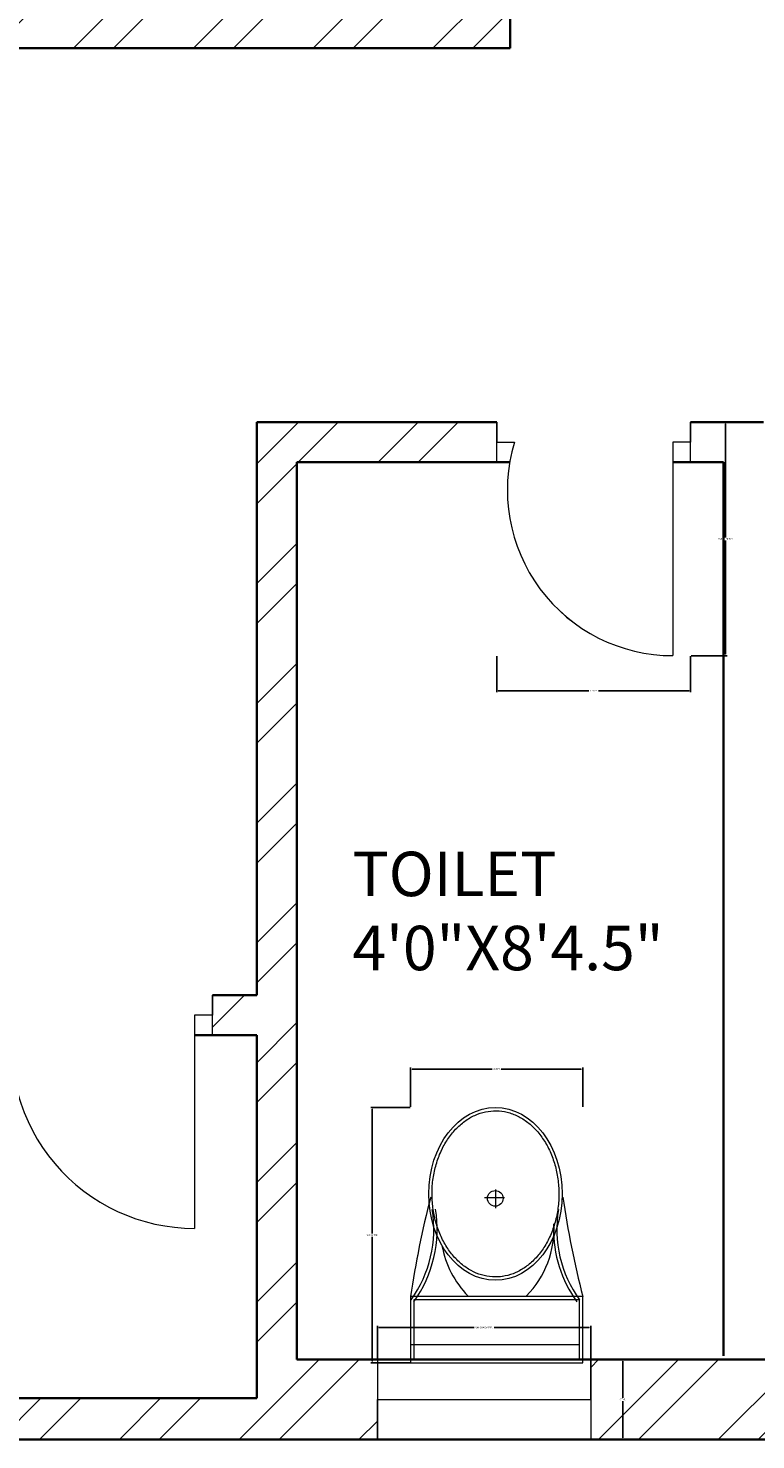
# Model space of a CAD drawing. Units: inches. Extents: x 2120 to 4013, y 1390 to 3019.
# Tile 3 of 59: x 2366 to 2448, y 1582 to 1740. Entities that reach past the tile are written whole.
import ezdxf

# ---------------------------------------------------------------- set-up
doc = ezdxf.new("R2010")
doc.units = ezdxf.units.IN
for name, color, linetype, lineweight in [('A-ANNO-DIMS', 2, 'Continuous', 18), ('A-AREA-IDEN', 7, 'Continuous', 18), ('A-DOOR', 3, 'Continuous', 18), ('A-FLOR-FIXT', 9, 'Continuous', 18), ('A-GLAZ', 4, 'Continuous', 18), ('A-WALL', 7, 'Continuous', 35), ('A-WALL-PATT', 252, 'Continuous', 13)]:
    doc.layers.add(name, color=color, linetype=linetype, lineweight=lineweight)
doc.styles.get("Standard").update_dxf_attribs({"font": 'arial.ttf'})
doc.dimstyles.get("Standard").update_dxf_attribs({"dimtxt": 0.18, "dimasz": 0.18, "dimexe": 0.18, "dimexo": 0.0625, "dimgap": 0.09, "dimtad": 0, "dimtih": 1, "dimtoh": 1, "dimdec": 4, "dimzin": 0, "dimdsep": 46, "dimtxsty": 'Standard', "dimcen": 0.09, "dimadec": 0, "dimazin": 0, "dimtfac": 1, "dimtdec": 4, "dimtofl": 0, "dimtmove": 0, "dimatfit": 3, "dimfxl": 1, "dimtolj": 1, "dimtzin": 0, "dimarcsym": 0})

# ---------------------------------------------------------------- blocks, each defined once
blk = doc.blocks.new('A$C31115884')
for p, q in [((257.5, 466.4), (257.5, 523.2)), ((283.1, 497.7), (223.4, 497.7)), ((0, 200), (0, 0)), ((520, 200), (0, 200)), ((10, 190), (10, 10)), ((510, 190), (10, 190)), ((510, 10), (510, 190)), ((520, 0), (520, 200)), ((510, 54.5), (0, 54.5)), ((10, 10), (510, 10)), ((0, 0), (520, 0))]:
    blk.add_line(p, q)
blk.add_circle((255.6, 496.4), 23.6)
for centre, radius, start, end in [((2777.7, -204.6), 2807, 165.4549, 171.7133), ((3237, 905), 2807, 188.2867, 194.5451), ((-294.5, 403.3), 364.7, 324.2091, 9.3499), ((-294.5, 403.3), 374.7, 324.2091, 9.3499), ((805.8, 403.3), 364.7, 170.6501, 215.7909), ((139.5, 406.2), 293.5, 315.8436, 2.6563), ((805.8, 403.3), 374.7, 179.2036, 215.7909), ((383.6, 406.2), 293.5, 190.2774, 224.1564)]:
    blk.add_arc(centre, radius, start, end)
blk.add_ellipse((256.2, 509.9), major_axis=(0, -260.7), ratio=0.772727)
blk.add_open_spline([(256.2, 259.2), (263.1, 259.2), (270, 259.7), (287.8, 262.3), (298.7, 265.1), (319.9, 273.1), (330.2, 278.4), (350.1, 291.1), (359.7, 298.7), (377.7, 315.9), (386.2, 325.5), (401.7, 346.6), (408.8, 358.1), (421.3, 382.5), (426.8, 395.5), (435.9, 422.4), (439.5, 436.4), (444.8, 465.1), (446.5, 479.7), (447.9, 509.2), (447.6, 524), (445, 553.3), (442.7, 567.8), (436.3, 596), (432.1, 609.7), (421.9, 636), (416, 648.6), (402.5, 672.1), (395, 683), (378.6, 703), (369.8, 712.1), (351.1, 728), (341.3, 734.8), (320.9, 746.2), (310.4, 750.7), (288.9, 757.3), (278, 759.4), (256, 761), (245, 760.6), (223.1, 757.2), (212.3, 754.3), (191.1, 746.1), (180.8, 740.7), (160.9, 727.8), (151.4, 720.1), (133.5, 702.7), (125.1, 693), (109.6, 671.7), (102.6, 660.2), (90.2, 635.7), (84.9, 622.7), (76, 595.6), (72.4, 581.6), (67.2, 552.9), (65.6, 538.2), (64.4, 508.8), (64.8, 494), (67.5, 464.7), (69.9, 450.2), (76.6, 422), (80.8, 408.3), (91.1, 382.2), (97.2, 369.7), (110.8, 346.3), (118.4, 335.4), (134.8, 315.6), (143.7, 306.7), (162.4, 290.9), (172.3, 284.2), (192.8, 273), (203.3, 268.6), (224.8, 262.2), (235.8, 260.2), (249.9, 259.3), (253, 259.2), (256.2, 259.2)], degree=3, knots=[0, 0, 0, 0, 0.110105, 0.110105, 0.285049, 0.285049, 0.459994, 0.459994, 0.634938, 0.634938, 0.809882, 0.809882, 0.984827, 0.984827, 1.159771, 1.159771, 1.334715, 1.334715, 1.50966, 1.50966, 1.684604, 1.684604, 1.859549, 1.859549, 2.034493, 2.034493, 2.209437, 2.209437, 2.384382, 2.384382, 2.559326, 2.559326, 2.73427, 2.73427, 2.909215, 2.909215, 3.084159, 3.084159, 3.259103, 3.259103, 3.434048, 3.434048, 3.608992, 3.608992, 3.783936, 3.783936, 3.958881, 3.958881, 4.133825, 4.133825, 4.30877, 4.30877, 4.483714, 4.483714, 4.658658, 4.658658, 4.833603, 4.833603, 5.008547, 5.008547, 5.183491, 5.183491, 5.358436, 5.358436, 5.53338, 5.53338, 5.708324, 5.708324, 5.883269, 5.883269, 6.058213, 6.058213, 6.233158, 6.233158, 6.283185, 6.283185, 6.283185, 6.283185])
blk = doc.blocks.new('DOOR-SWING-24IN-106p83DEG')
for p, q in [((0, 21.75), (0, 26.25)), ((0, 26.25), (0, 24)), ((21.81, 21.75), (21.81, 26.25)), ((21.81, 26.25), (21.81, 24)), ((0, 24), (2, 24)), ((21.81, 24), (19.81, 24)), ((19.81, 24), (19.81, 0))]:
    blk.add_line(p, q)
blk.add_arc((19.81, 18.61), 18.61, 163.1661, 270)
blk = doc.blocks.new('DOOR-SWING-24IN-99p42DEG')
for p, q in [((0, 26.25), (0, 21.75)), ((24.35, 21.75), (24.35, 26.25)), ((24.35, 26.25), (24.35, 24)), ((0, 21.75), (0, 24)), ((0, 24), (2, 24)), ((24.35, 24), (22.35, 24)), ((22.35, 24), (22.35, 0))]:
    blk.add_line(p, q)
blk.add_arc((22.35, 20.62), 20.62, 170.5813, 270)
blk = doc.blocks.new('WIN-PLAN-24IN-03')
for p, q in [((9, 24), (0, 24)), ((0, 24), (4.5, 24)), ((4.5, 24), (4.5, 0)), ((9, 0), (0, 0)), ((4.5, 0), (9, 0))]:
    blk.add_line(p, q)
blk = doc.blocks.new('*D71')
at = {"layer": 'A-ANNO-DIMS', "color": 0, "lineweight": -2, "transparency": 16777216}
for p, q in [((2408.97, 1618.88), (2404.55, 1618.88)), ((2404.73, 1618.7), (2404.73, 1604.7)), ((2404.73, 1590.34), (2404.73, 1604.34)), ((2408.97, 1590.16), (2404.55, 1590.16))]:
    blk.add_line(p, q, dxfattribs=at)
at = {"layer": 'A-ANNO-DIMS', "color": 0, "transparency": 16777216}
for points in [[(2404.7, 1618.7), (2404.76, 1618.7), (2404.73, 1618.88)], [(2404.7, 1590.34), (2404.76, 1590.34), (2404.73, 1590.16)]]:
    blk.add_solid(points, dxfattribs=at)
at = {"layer": 'Defpoints', "color": 0, "transparency": 16777216}
for p in [(2404.73, 1618.88), (2409.03, 1618.88), (2409.03, 1590.16)]:
    blk.add_point(p, dxfattribs=at)
at = {"layer": 'A-ANNO-DIMS', "color": 0, "transparency": 16777216, "insert": (2404.73, 1604.52), "char_height": 0.18, "attachment_point": 5}
blk.add_mtext('\\A1;WC 29 TYP.', dxfattribs=at)
blk = doc.blocks.new('*D72')
at = {"layer": 'A-ANNO-DIMS', "color": 0, "lineweight": -2, "transparency": 16777216}
for p, q in [((2409.03, 1618.94), (2409.03, 1623.37)), ((2409.21, 1623.19), (2418.2, 1623.19)), ((2428.23, 1623.19), (2419.24, 1623.19)), ((2428.41, 1618.94), (2428.41, 1623.37))]:
    blk.add_line(p, q, dxfattribs=at)
at = {"layer": 'A-ANNO-DIMS', "color": 0, "transparency": 16777216}
for points in [[(2409.21, 1623.22), (2409.21, 1623.16), (2409.03, 1623.19)], [(2428.23, 1623.22), (2428.23, 1623.16), (2428.41, 1623.19)]]:
    blk.add_solid(points, dxfattribs=at)
at = {"layer": 'Defpoints', "color": 0, "transparency": 16777216}
for p in [(2428.41, 1623.19), (2409.03, 1618.88), (2428.41, 1618.88)]:
    blk.add_point(p, dxfattribs=at)
at = {"layer": 'A-ANNO-DIMS', "color": 0, "transparency": 16777216, "insert": (2418.72, 1623.19), "char_height": 0.18, "attachment_point": 5}
blk.add_mtext('\\A1;19 TYP.', dxfattribs=at)
blk = doc.blocks.new('*D139')
at = {"layer": 'A-ANNO-DIMS', "color": 0, "lineweight": -2, "transparency": 16777216}
for p, q in [((2440.6, 1695.95), (2444.65, 1695.95)), ((2444.47, 1695.77), (2444.47, 1683.01)), ((2444.47, 1669.88), (2444.47, 1682.64)), ((2440.6, 1669.7), (2444.65, 1669.7))]:
    blk.add_line(p, q, dxfattribs=at)
at = {"layer": 'A-ANNO-DIMS', "color": 0, "transparency": 16777216}
for points in [[(2444.44, 1695.77), (2444.5, 1695.77), (2444.47, 1695.95)], [(2444.44, 1669.88), (2444.5, 1669.88), (2444.47, 1669.7)]]:
    blk.add_solid(points, dxfattribs=at)
at = {"layer": 'Defpoints', "color": 0, "transparency": 16777216}
for p in [(2440.53, 1695.95), (2444.47, 1695.95), (2440.53, 1669.7)]:
    blk.add_point(p, dxfattribs=at)
at = {"layer": 'A-ANNO-DIMS', "color": 0, "transparency": 16777216, "insert": (2444.47, 1682.83), "char_height": 0.18, "attachment_point": 5}
blk.add_mtext('\\A1;SWING 26 TYP.', dxfattribs=at)
blk = doc.blocks.new('*D140')
at = {"layer": 'A-ANNO-DIMS', "color": 0, "lineweight": -2, "transparency": 16777216}
for p, q in [((2418.72, 1669.64), (2418.72, 1665.58)), ((2440.53, 1669.64), (2440.53, 1665.58)), ((2418.9, 1665.76), (2429.1, 1665.76)), ((2440.35, 1665.76), (2430.16, 1665.76))]:
    blk.add_line(p, q, dxfattribs=at)
at = {"layer": 'A-ANNO-DIMS', "color": 0, "transparency": 16777216}
for points in [[(2418.9, 1665.79), (2418.9, 1665.73), (2418.72, 1665.76)], [(2440.35, 1665.79), (2440.35, 1665.73), (2440.53, 1665.76)]]:
    blk.add_solid(points, dxfattribs=at)
at = {"layer": 'Defpoints', "color": 0, "transparency": 16777216}
for p in [(2418.72, 1669.7), (2440.53, 1669.7), (2440.53, 1665.76)]:
    blk.add_point(p, dxfattribs=at)
at = {"layer": 'A-ANNO-DIMS', "color": 0, "transparency": 16777216, "insert": (2429.63, 1665.76), "char_height": 0.18, "attachment_point": 5}
blk.add_mtext('\\A1;22 TYP.', dxfattribs=at)
blk = doc.blocks.new('*D169')
at = {"layer": 'A-ANNO-DIMS', "color": 0, "lineweight": -2, "transparency": 16777216}
for p, q in [((2405.3, 1590.59), (2405.3, 1594.31)), ((2405.48, 1594.13), (2416.18, 1594.13)), ((2429.12, 1594.13), (2418.42, 1594.13)), ((2429.3, 1590.59), (2429.3, 1594.31))]:
    blk.add_line(p, q, dxfattribs=at)
at = {"layer": 'A-ANNO-DIMS', "color": 0, "transparency": 16777216}
for points in [[(2405.48, 1594.16), (2405.48, 1594.1), (2405.3, 1594.13)], [(2429.12, 1594.16), (2429.12, 1594.1), (2429.3, 1594.13)]]:
    blk.add_solid(points, dxfattribs=at)
at = {"layer": 'Defpoints', "color": 0, "transparency": 16777216}
for p in [(2405.3, 1594.13), (2405.3, 1590.53), (2429.3, 1590.53)]:
    blk.add_point(p, dxfattribs=at)
at = {"layer": 'A-ANNO-DIMS', "color": 0, "transparency": 16777216, "insert": (2417.3, 1594.13), "char_height": 0.18, "attachment_point": 5}
blk.add_mtext('\\A1;WINDOW 24 TYP.', dxfattribs=at)
blk = doc.blocks.new('*D170')
at = {"layer": 'A-ANNO-DIMS', "color": 0, "lineweight": -2, "transparency": 16777216}
for p, q in [((2429.37, 1590.53), (2433.08, 1590.53)), ((2432.9, 1590.35), (2432.9, 1586.21)), ((2432.9, 1581.71), (2432.9, 1585.85)), ((2429.37, 1581.53), (2433.08, 1581.53))]:
    blk.add_line(p, q, dxfattribs=at)
at = {"layer": 'A-ANNO-DIMS', "color": 0, "transparency": 16777216}
for points in [[(2432.87, 1590.35), (2432.93, 1590.35), (2432.9, 1590.53)], [(2432.87, 1581.71), (2432.93, 1581.71), (2432.9, 1581.53)]]:
    blk.add_solid(points, dxfattribs=at)
at = {"layer": 'Defpoints', "color": 0, "transparency": 16777216}
for p in [(2429.3, 1590.53), (2432.9, 1590.53), (2429.3, 1581.53)]:
    blk.add_point(p, dxfattribs=at)
at = {"layer": 'A-ANNO-DIMS', "color": 0, "transparency": 16777216, "insert": (2432.9, 1586.03), "char_height": 0.18, "attachment_point": 5}
blk.add_mtext('\\A1;9 TYP.', dxfattribs=at)

msp = doc.modelspace()

# ---------------------------------------------------------------- hatches: boundary and pattern name
at = {"layer": 'A-WALL-PATT'}
h = msp.add_hatch(dxfattribs=at)
h.set_pattern_fill('ANSI32', color=256)
h.paths.add_polyline_path([(2271.7331, 2343.531), (2283.3788, 2343.531), (2283.3788, 2348.031), (2283.3788, 2352.5306), (2262.7331, 2352.5306), (2262.7331, 2182.638), (2267.2331, 2182.638), (2271.7331, 2182.638), (2271.7331, 2219.031), (2391.7331, 2219.031), (2391.7331, 2214.189), (2393.9831, 2214.189), (2396.2331, 2214.189), (2396.2331, 2219.031), (2420.2331, 2219.031), (2420.2331, 2225.7535), (2417.2197, 2225.7535), (2415.7331, 2225.7535), (2415.7331, 2223.5306), (2271.7331, 2223.5306)])
h.paths.add_polyline_path([(2380.0942, 2352.5306), (2343.3788, 2352.5306), (2343.3788, 2343.531), (2363.2331, 2343.531), (2363.2331, 2288.8489), (2365.4831, 2288.8489), (2367.7331, 2288.8489), (2367.7331, 2343.531), (2380.0942, 2343.531)], flags=17)
h.paths.add_polyline_path([(2432.4339, 2352.5306), (2404.0943, 2352.5306), (2404.0943, 2343.531), (2415.7331, 2343.531), (2415.7331, 2264.0306), (2367.7331, 2264.0306), (2367.7331, 2266.4872), (2363.2331, 2266.4872), (2363.2331, 2259.531), (2367.7331, 2259.531), (2415.7331, 2259.531), (2415.7331, 2255.0658), (2420.2331, 2255.0658), (2420.2331, 2259.531), (2424.5717, 2259.531), (2424.5717, 2261.781), (2424.5717, 2264.0306), (2420.2331, 2264.0306), (2420.2331, 2343.531), (2432.4339, 2343.531)])
h.paths.add_polyline_path([(2508.9115, 2352.5306), (2456.4339, 2352.5306), (2456.4339, 2343.531), (2468.2331, 2343.531), (2468.2331, 2264.0306), (2448.0487, 2264.0306), (2448.0487, 2259.531), (2468.2331, 2259.531), (2468.2331, 2255.5496), (2472.7331, 2255.5496), (2472.7331, 2343.531), (2508.9115, 2343.531)])
h.paths.add_polyline_path([(2637.7331, 2352.5306), (2544.9116, 2352.5306), (2544.9116, 2343.531), (2589.7331, 2343.531), (2633.2331, 2343.531), (2637.7331, 2343.531)])
h.paths.add_polyline_path([(2594.2331, 2343.5306), (2589.7331, 2343.5306), (2589.7331, 2259.5306), (2589.7331, 2252.4915), (2591.9831, 2252.4915), (2594.2331, 2252.4915)])
h.paths.add_polyline_path([(2637.7331, 2223.5306), (2594.2331, 2223.5306), (2594.2331, 2230.1988), (2591.9831, 2230.1988), (2589.7331, 2230.1988), (2589.7331, 2223.5306), (2472.7331, 2223.5306), (2468.2331, 2223.5306), (2468.2331, 2219.031), (2628.7331, 2219.031), (2628.7331, 2138.031), (2637.7331, 2138.031)])
h.paths.add_polyline_path([(3822.6535, 2458.4402), (3874.9468, 2458.4402), (3874.9468, 2476.9866), (3822.6535, 2476.9866)], flags=9)
h.paths.add_polyline_path([(3834.6921, 2781.8174), (3935.9206, 2781.8174), (3935.9206, 2800.3638), (3834.6921, 2800.3638)], flags=9)
h.paths.add_polyline_path([(3832.2843, 2837.9683), (3884.5776, 2837.9683), (3884.5776, 2856.5146), (3832.2843, 2856.5146)], flags=9)
h.paths.add_polyline_path([(3830.9388, 2861.4782), (3956.8958, 2861.4782), (3956.8958, 2880.0245), (3830.9388, 2880.0245)], flags=9)
h.paths.add_polyline_path([(3870.6966, 2352.5752), (3887.9272, 2352.5752), (3887.9272, 2377.3037), (3870.6966, 2377.3037)], flags=9)
h.paths.add_polyline_path([(3289.2701, 2413.161), (3435.2223, 2413.161), (3435.2223, 2450.2538), (3289.2701, 2450.2538)], flags=9)
h.paths.add_polyline_path([(2487.6944, 2414.3601), (2637.8335, 2414.3601), (2637.8335, 2451.4528), (2487.6944, 2451.4528)], flags=9)
h.paths.add_polyline_path([(2567.3724, 1457.9199), (2815.296, 1457.9199), (2815.296, 1495.0127), (2567.3724, 1495.0127)], flags=9)
h.paths.add_polyline_path([(2655.3825, 2093.2363), (2685.9555, 2093.2363), (2685.9555, 2111.8937), (2655.3825, 2111.8937)], flags=9)
h.paths.add_polyline_path([(2543.9218, 1550.6671), (2587.8406, 1550.6671), (2587.8406, 1569.3244), (2543.9218, 1569.3244)], flags=9)
h.paths.add_polyline_path([(2905.1384, 1543.8113), (2949.0572, 1543.8113), (2949.0572, 1562.4686), (2905.1384, 1562.4686)], flags=9)
h.paths.add_polyline_path([(2736.4118, 1702.4736), (2784.2153, 1702.4736), (2784.2153, 1721.1309), (2736.4118, 1721.1309)], flags=9)
h.paths.add_polyline_path([(2912.8666, 1710.4168), (2951.707, 1710.4168), (2951.707, 1729.0741), (2912.8666, 1729.0741)], flags=9)
h.paths.add_polyline_path([(2923.5785, 1763.5038), (2959.7279, 1763.5038), (2959.7279, 1782.1611), (2923.5785, 1782.1611)], flags=9)
h.paths.add_polyline_path([(2925.2114, 1809.6137), (2967.1861, 1809.6137), (2967.1861, 1828.271), (2925.2114, 1828.271)], flags=9)
h.paths.add_polyline_path([(2996.2711, 1878.9003), (2996.2711, 1913.109), (2977.6138, 1913.109), (2977.6138, 1878.9003)], flags=9)
h.paths.add_polyline_path([(2883.0859, 1895.7192), (2927.1855, 1895.7192), (2927.1855, 1914.3766), (2883.0859, 1914.3766)], flags=9)
h.paths.add_polyline_path([(2787.3924, 1810.8013), (2841.0213, 1810.8013), (2841.0213, 1829.4587), (2787.3924, 1829.4587)], flags=9)
h.paths.add_polyline_path([(2775.6399, 2101.7395), (2829.2689, 2101.7395), (2829.2689, 2120.3968), (2775.6399, 2120.3968)], flags=9)
h.paths.add_polyline_path([(2913.0263, 2075.817), (2951.8667, 2075.817), (2951.8667, 2094.4744), (2913.0263, 2094.4744)], flags=9)
h.paths.add_polyline_path([(2929.966, 2133.3669), (2966.1154, 2133.3669), (2966.1154, 2152.0243), (2929.966, 2152.0243)], flags=9)
h.paths.add_polyline_path([(2932.7502, 2182.6088), (2968.8996, 2182.6088), (2968.8996, 2201.2662), (2932.7502, 2201.2662)], flags=9)
h.paths.add_polyline_path([(2996.0681, 2266.3173), (2996.0681, 2300.5261), (2977.4108, 2300.5261), (2977.4108, 2266.3173)], flags=9)
h.paths.add_polyline_path([(2885.1039, 2279.2186), (2929.2035, 2279.2186), (2929.2035, 2297.8759), (2885.1039, 2297.8759)], flags=9)
h.paths.add_polyline_path([(2735.7042, 2218.3197), (2783.5078, 2218.3197), (2783.5078, 2236.9771), (2735.7042, 2236.9771)], flags=9)
h.paths.add_polyline_path([(2635.6049, 2044.0085), (2648.9678, 2044.0085), (2648.9678, 2054.312), (2635.6049, 2054.312)], flags=9)
h.paths.add_polyline_path([(2714.0148, 1923.0473), (2727.3777, 1923.0473), (2727.3777, 1933.3508), (2714.0148, 1933.3508)], flags=9)
h.paths.add_polyline_path([(2709.0345, 1988.1628), (2722.3974, 1988.1628), (2722.3974, 1998.4663), (2709.0345, 1998.4663)], flags=9)
h.paths.add_polyline_path([(2592.8935, 1962.1763), (2606.2564, 1962.1763), (2606.2564, 1972.4799), (2592.8935, 1972.4799)], flags=9)
h.paths.add_polyline_path([(2618.3996, 1985.9724), (2644.1942, 1985.9724), (2644.1942, 1996.2759), (2618.3996, 1996.2759)], flags=9)
h.paths.add_polyline_path([(2601.279, 1920.5869), (2614.6419, 1920.5869), (2614.6419, 1930.8904), (2601.279, 1930.8904)], flags=9)
h.paths.add_polyline_path([(2692.3278, 1932.7645), (2704.5311, 1932.7645), (2704.5311, 1943.0681), (2692.3278, 1943.0681)], flags=9)
h.paths.add_polyline_path([(2311.122, 1672.7318), (2355.0408, 1672.7318), (2355.0408, 1691.3892), (2311.122, 1691.3892)], flags=9)
h.paths.add_polyline_path([(2456.2551, 1632.3198), (2492.4796, 1632.3198), (2492.4796, 1650.9772), (2456.2551, 1650.9772)], flags=9)
h.paths.add_polyline_path([(2401.0766, 1631.4793), (2437.301, 1631.4793), (2437.301, 1650.1367), (2401.0766, 1650.1367)], flags=9)
h.paths.add_polyline_path([(2546.7054, 1700.9235), (2594.509, 1700.9235), (2594.509, 1719.5809), (2546.7054, 1719.5809)], flags=9)
h.paths.add_polyline_path([(2445.4866, 1766.9937), (2497.5261, 1766.9937), (2497.5261, 1785.651), (2445.4866, 1785.651)], flags=9)
h.paths.add_polyline_path([(2287.9992, 1739.7675), (2326.8396, 1739.7675), (2326.8396, 1758.4248), (2287.9992, 1758.4248)], flags=9)
h.paths.add_polyline_path([(2458.5279, 1924.7607), (2510.5675, 1924.7607), (2510.5675, 1943.4181), (2458.5279, 1943.4181)], flags=9)
h.paths.add_polyline_path([(2309.2811, 1902.7642), (2345.4305, 1902.7642), (2345.4305, 1921.4215), (2309.2811, 1921.4215)], flags=9)
h.paths.add_polyline_path([(2490.7554, 2018.9392), (2530.7896, 2018.9392), (2530.7896, 2037.5965), (2490.7554, 2037.5965)], flags=9)
h.paths.add_polyline_path([(2402.143, 2024.7393), (2438.5414, 2024.7393), (2438.5414, 2043.3966), (2402.143, 2043.3966)], flags=9)
h.paths.add_polyline_path([(2287.856, 1931.7926), (2326.6964, 1931.7926), (2326.6964, 1950.4499), (2287.856, 1950.4499)], flags=9)
h.paths.add_polyline_path([(2281.7979, 2193.5771), (2320.6383, 2193.5771), (2320.6383, 2212.2344), (2281.7979, 2212.2344)], flags=25)
h.paths.add_polyline_path([(2484.0754, 2093.892), (2536.115, 2093.892), (2536.115, 2112.5494), (2484.0754, 2112.5494)], flags=9)
h.paths.add_polyline_path([(2624.7948, 2281.8639), (2624.7948, 2311.4137), (2606.1375, 2311.4137), (2606.1375, 2281.8639)], flags=9)
h.paths.add_polyline_path([(2507.5036, 2290.3639), (2541.934, 2290.3639), (2541.934, 2309.0212), (2507.5036, 2309.0212)], flags=9)
h.paths.add_polyline_path([(2423.1076, 2285.2202), (2459.332, 2285.2202), (2459.332, 2303.8776), (2423.1076, 2303.8776)], flags=9)
h.paths.add_polyline_path([(2374.5467, 2289.6272), (2410.7711, 2289.6272), (2410.7711, 2308.2846), (2374.5467, 2308.2846)], flags=25)
h.paths.add_polyline_path([(2277.4907, 2227.5651), (2316.3311, 2227.5651), (2316.3311, 2246.2224), (2277.4907, 2246.2224)], flags=25)
h.paths.add_polyline_path([(2655.3825, 2093.2367), (2685.9555, 2093.2367), (2685.9555, 2111.894), (2655.3825, 2111.894)], flags=9)
h.paths.add_polyline_path([(2543.9217, 1550.6674), (2587.8406, 1550.6674), (2587.8406, 1569.3247), (2543.9217, 1569.3247)], flags=9)
h.paths.add_polyline_path([(2905.1384, 1543.8116), (2949.0572, 1543.8116), (2949.0572, 1562.4689), (2905.1384, 1562.4689)], flags=9)
h.paths.add_polyline_path([(2736.4118, 1702.4739), (2784.2153, 1702.4739), (2784.2153, 1721.1312), (2736.4118, 1721.1312)], flags=9)
h.paths.add_polyline_path([(2912.8666, 1710.4171), (2951.707, 1710.4171), (2951.707, 1729.0744), (2912.8666, 1729.0744)], flags=9)
h.paths.add_polyline_path([(2923.5785, 1763.5041), (2959.7279, 1763.5041), (2959.7279, 1782.1614), (2923.5785, 1782.1614)], flags=9)
h.paths.add_polyline_path([(2925.2114, 1809.614), (2967.1861, 1809.614), (2967.1861, 1828.2713), (2925.2114, 1828.2713)], flags=9)
h.paths.add_polyline_path([(2996.2711, 1878.9006), (2996.2711, 1913.1094), (2977.6137, 1913.1094), (2977.6137, 1878.9006)], flags=9)
h.paths.add_polyline_path([(2883.0859, 1895.7195), (2927.1855, 1895.7195), (2927.1855, 1914.3769), (2883.0859, 1914.3769)], flags=9)
h.paths.add_polyline_path([(2787.3924, 1810.8016), (2841.0213, 1810.8016), (2841.0213, 1829.459), (2787.3924, 1829.459)], flags=9)
h.paths.add_polyline_path([(2775.6399, 2101.7398), (2829.2688, 2101.7398), (2829.2688, 2120.3971), (2775.6399, 2120.3971)], flags=9)
h.paths.add_polyline_path([(2913.0263, 2075.8173), (2951.8667, 2075.8173), (2951.8667, 2094.4747), (2913.0263, 2094.4747)], flags=9)
h.paths.add_polyline_path([(2929.966, 2133.3672), (2966.1154, 2133.3672), (2966.1154, 2152.0246), (2929.966, 2152.0246)], flags=9)
h.paths.add_polyline_path([(2932.7502, 2182.6091), (2968.8996, 2182.6091), (2968.8996, 2201.2665), (2932.7502, 2201.2665)], flags=9)
h.paths.add_polyline_path([(2996.0681, 2266.3176), (2996.0681, 2300.5264), (2977.4108, 2300.5264), (2977.4108, 2266.3176)], flags=9)
h.paths.add_polyline_path([(2885.1039, 2279.2189), (2929.2035, 2279.2189), (2929.2035, 2297.8762), (2885.1039, 2297.8762)], flags=9)
h.paths.add_polyline_path([(2735.7042, 2218.32), (2783.5078, 2218.32), (2783.5078, 2236.9774), (2735.7042, 2236.9774)], flags=9)
h.paths.add_polyline_path([(2635.6048, 2044.0088), (2648.9677, 2044.0088), (2648.9677, 2054.3123), (2635.6048, 2054.3123)], flags=9)
h.paths.add_polyline_path([(2714.0148, 1923.0476), (2727.3777, 1923.0476), (2727.3777, 1933.3511), (2714.0148, 1933.3511)], flags=9)
h.paths.add_polyline_path([(2709.0345, 1988.1631), (2722.3974, 1988.1631), (2722.3974, 1998.4666), (2709.0345, 1998.4666)], flags=9)
h.paths.add_polyline_path([(2592.8935, 1962.1766), (2606.2564, 1962.1766), (2606.2564, 1972.4802), (2592.8935, 1972.4802)], flags=9)
h.paths.add_polyline_path([(2618.3995, 1985.9727), (2644.1942, 1985.9727), (2644.1942, 1996.2762), (2618.3995, 1996.2762)], flags=9)
h.paths.add_polyline_path([(2601.279, 1920.5872), (2614.6419, 1920.5872), (2614.6419, 1930.8908), (2601.279, 1930.8908)], flags=9)
h.paths.add_polyline_path([(2692.3278, 1932.7648), (2704.5311, 1932.7648), (2704.5311, 1943.0684), (2692.3278, 1943.0684)], flags=9)
h.paths.add_polyline_path([(2311.122, 1672.7321), (2355.0408, 1672.7321), (2355.0408, 1691.3895), (2311.122, 1691.3895)], flags=9)
h.paths.add_polyline_path([(2456.2551, 1632.3201), (2492.4795, 1632.3201), (2492.4795, 1650.9775), (2456.2551, 1650.9775)], flags=9)
h.paths.add_polyline_path([(2401.0766, 1631.4796), (2437.301, 1631.4796), (2437.301, 1650.137), (2401.0766, 1650.137)], flags=9)
h.paths.add_polyline_path([(2546.7054, 1700.9238), (2594.509, 1700.9238), (2594.509, 1719.5812), (2546.7054, 1719.5812)], flags=9)
h.paths.add_polyline_path([(2445.4866, 1766.994), (2497.5261, 1766.994), (2497.5261, 1785.6513), (2445.4866, 1785.6513)], flags=9)
h.paths.add_polyline_path([(2287.9992, 1739.7678), (2326.8396, 1739.7678), (2326.8396, 1758.4251), (2287.9992, 1758.4251)], flags=9)
h.paths.add_polyline_path([(2458.5279, 1924.7611), (2510.5675, 1924.7611), (2510.5675, 1943.4184), (2458.5279, 1943.4184)], flags=9)
h.paths.add_polyline_path([(2309.2811, 1902.7645), (2345.4305, 1902.7645), (2345.4305, 1921.4218), (2309.2811, 1921.4218)], flags=9)
h.paths.add_polyline_path([(2490.7554, 2018.9395), (2530.7895, 2018.9395), (2530.7895, 2037.5968), (2490.7554, 2037.5968)], flags=9)
h.paths.add_polyline_path([(2402.143, 2024.7396), (2438.5413, 2024.7396), (2438.5413, 2043.3969), (2402.143, 2043.3969)], flags=9)
h.paths.add_polyline_path([(2287.856, 1931.7929), (2326.6964, 1931.7929), (2326.6964, 1950.4502), (2287.856, 1950.4502)], flags=9)
h.paths.add_polyline_path([(2281.7979, 2193.5774), (2320.6383, 2193.5774), (2320.6383, 2212.2347), (2281.7979, 2212.2347)], flags=25)
h.paths.add_polyline_path([(2484.0754, 2093.8924), (2536.115, 2093.8924), (2536.115, 2112.5497), (2484.0754, 2112.5497)], flags=9)
h.paths.add_polyline_path([(2624.7948, 2281.8642), (2624.7948, 2311.414), (2606.1374, 2311.414), (2606.1374, 2281.8642)], flags=9)
h.paths.add_polyline_path([(2507.5035, 2290.3642), (2541.934, 2290.3642), (2541.934, 2309.0215), (2507.5035, 2309.0215)], flags=9)
h.paths.add_polyline_path([(2423.1075, 2285.2205), (2459.332, 2285.2205), (2459.332, 2303.8779), (2423.1075, 2303.8779)], flags=9)
h.paths.add_polyline_path([(2374.5467, 2289.6275), (2410.7711, 2289.6275), (2410.7711, 2308.2849), (2374.5467, 2308.2849)], flags=25)
h.paths.add_polyline_path([(2277.4907, 2227.5654), (2316.3311, 2227.5654), (2316.3311, 2246.2227), (2277.4907, 2246.2227)], flags=25)
h = msp.add_hatch(dxfattribs=at)
h.set_pattern_fill('ANSI32', color=256)
h.paths.add_polyline_path([(2271.7331, 1980.389), (2262.7331, 1980.389), (2262.7331, 1912.8434), (2267.2331, 1912.8434), (2271.7331, 1912.8434), (2271.7331, 1922.531), (2351.2331, 1922.531), (2351.2331, 1901.4728), (2355.7331, 1901.4728), (2355.7331, 1922.531), (2357.9815, 1922.531), (2357.9815, 1926.5306), (2271.7331, 1926.5306)])
h.paths.add_polyline_path([(2589.2331, 1949.1622), (2584.7331, 1949.1622), (2580.2331, 1949.1622), (2580.2331, 1874.5306), (2355.7331, 1874.5306), (2355.7331, 1880.1922), (2351.2331, 1880.1922), (2351.2331, 1874.5306), (2271.7331, 1874.5306), (2271.7331, 1888.8431), (2262.7331, 1888.8431), (2262.7331, 1842.2909), (2267.2331, 1842.2909), (2271.7331, 1842.2909), (2271.7331, 1865.531), (2415.7331, 1865.531), (2415.7331, 1779.7286), (2420.2331, 1779.7286), (2420.2331, 1865.531), (2589.2331, 1865.531)])
h.paths.add_polyline_path([(2271.7331, 1782.2906), (2262.7331, 1782.2906), (2262.7331, 1711.4639), (2267.2331, 1711.4639), (2271.7331, 1711.4639), (2271.7331, 1738.031), (2420.2331, 1738.031), (2420.2331, 1742.531), (2420.2331, 1747.3376), (2417.9831, 1747.3376), (2415.7331, 1747.3376), (2415.7331, 1742.5306), (2271.7331, 1742.5306)])
h.paths.add_polyline_path([(2271.7331, 1627.031), (2362.3957, 1627.031), (2362.3957, 1629.281), (2362.3957, 1631.5306), (2271.7331, 1631.5306), (2271.7331, 1675.4636), (2262.7331, 1675.4636), (2262.7331, 1581.531), (2405.3032, 1581.531), (2405.3032, 1586.031), (2405.3032, 1590.5306), (2396.2331, 1590.5306), (2396.2331, 1691.4513), (2418.7206, 1691.4513), (2418.7206, 1695.951), (2396.2331, 1695.951), (2391.7331, 1695.951), (2391.7331, 1631.5306), (2386.7425, 1631.5306), (2386.7425, 1629.2806), (2386.7425, 1627.031), (2391.7331, 1627.031), (2391.7331, 1586.1709), (2271.7331, 1586.1709)])
h.paths.add_polyline_path([(2459.6703, 1590.5306), (2429.3032, 1590.5306), (2429.3032, 1581.531), (2459.6703, 1581.531), (2459.6703, 1586.031)])
h.paths.add_polyline_path([(2501.2331, 1590.531), (2501.2331, 1665.0195), (2498.9831, 1665.0195), (2496.7331, 1665.0195), (2496.7331, 1590.5306), (2483.8201, 1590.5306), (2483.8201, 1590.1579), (2483.6704, 1590.1579), (2483.6704, 1581.531), (2505.0196, 1581.531), (2505.0196, 1583.781), (2505.0196, 1586.0306), (2501.2331, 1586.0306)])
h.paths.add_polyline_path([(2544.1361, 1583.781), (2544.1361, 1586.0306), (2527.1368, 1586.0306), (2527.1368, 1583.7806), (2527.1368, 1581.531), (2544.1361, 1581.531)])
h.paths.add_polyline_path([(3822.6535, 2458.4402), (3874.9468, 2458.4402), (3874.9468, 2476.9866), (3822.6535, 2476.9866)], flags=9)
h.paths.add_polyline_path([(3834.6921, 2781.8174), (3935.9206, 2781.8174), (3935.9206, 2800.3638), (3834.6921, 2800.3638)], flags=9)
h.paths.add_polyline_path([(3832.2843, 2837.9683), (3884.5776, 2837.9683), (3884.5776, 2856.5146), (3832.2843, 2856.5146)], flags=9)
h.paths.add_polyline_path([(3830.9388, 2861.4782), (3956.8958, 2861.4782), (3956.8958, 2880.0245), (3830.9388, 2880.0245)], flags=9)
h.paths.add_polyline_path([(3870.6966, 2352.5752), (3887.9272, 2352.5752), (3887.9272, 2377.3037), (3870.6966, 2377.3037)], flags=9)
h.paths.add_polyline_path([(3289.2701, 2413.161), (3435.2223, 2413.161), (3435.2223, 2450.2538), (3289.2701, 2450.2538)], flags=9)
h.paths.add_polyline_path([(2487.6944, 2414.3601), (2637.8335, 2414.3601), (2637.8335, 2451.4528), (2487.6944, 2451.4528)], flags=9)
h.paths.add_polyline_path([(2567.3724, 1457.9199), (2815.296, 1457.9199), (2815.296, 1495.0127), (2567.3724, 1495.0127)], flags=9)
h.paths.add_polyline_path([(2655.3825, 2093.2363), (2685.9555, 2093.2363), (2685.9555, 2111.8937), (2655.3825, 2111.8937)], flags=9)
h.paths.add_polyline_path([(2543.9218, 1550.6671), (2587.8406, 1550.6671), (2587.8406, 1569.3244), (2543.9218, 1569.3244)], flags=9)
h.paths.add_polyline_path([(2905.1384, 1543.8113), (2949.0572, 1543.8113), (2949.0572, 1562.4686), (2905.1384, 1562.4686)], flags=9)
h.paths.add_polyline_path([(2736.4118, 1702.4736), (2784.2153, 1702.4736), (2784.2153, 1721.1309), (2736.4118, 1721.1309)], flags=9)
h.paths.add_polyline_path([(2912.8666, 1710.4168), (2951.707, 1710.4168), (2951.707, 1729.0741), (2912.8666, 1729.0741)], flags=9)
h.paths.add_polyline_path([(2923.5785, 1763.5038), (2959.7279, 1763.5038), (2959.7279, 1782.1611), (2923.5785, 1782.1611)], flags=9)
h.paths.add_polyline_path([(2925.2114, 1809.6137), (2967.1861, 1809.6137), (2967.1861, 1828.271), (2925.2114, 1828.271)], flags=9)
h.paths.add_polyline_path([(2996.2711, 1878.9003), (2996.2711, 1913.109), (2977.6138, 1913.109), (2977.6138, 1878.9003)], flags=9)
h.paths.add_polyline_path([(2883.0859, 1895.7192), (2927.1855, 1895.7192), (2927.1855, 1914.3766), (2883.0859, 1914.3766)], flags=9)
h.paths.add_polyline_path([(2787.3924, 1810.8013), (2841.0213, 1810.8013), (2841.0213, 1829.4587), (2787.3924, 1829.4587)], flags=9)
h.paths.add_polyline_path([(2775.6399, 2101.7395), (2829.2689, 2101.7395), (2829.2689, 2120.3968), (2775.6399, 2120.3968)], flags=9)
h.paths.add_polyline_path([(2913.0263, 2075.817), (2951.8667, 2075.817), (2951.8667, 2094.4744), (2913.0263, 2094.4744)], flags=9)
h.paths.add_polyline_path([(2929.966, 2133.3669), (2966.1154, 2133.3669), (2966.1154, 2152.0243), (2929.966, 2152.0243)], flags=9)
h.paths.add_polyline_path([(2932.7502, 2182.6088), (2968.8996, 2182.6088), (2968.8996, 2201.2662), (2932.7502, 2201.2662)], flags=9)
h.paths.add_polyline_path([(2996.0681, 2266.3173), (2996.0681, 2300.5261), (2977.4108, 2300.5261), (2977.4108, 2266.3173)], flags=9)
h.paths.add_polyline_path([(2885.1039, 2279.2186), (2929.2035, 2279.2186), (2929.2035, 2297.8759), (2885.1039, 2297.8759)], flags=9)
h.paths.add_polyline_path([(2735.7042, 2218.3197), (2783.5078, 2218.3197), (2783.5078, 2236.9771), (2735.7042, 2236.9771)], flags=9)
h.paths.add_polyline_path([(2635.6049, 2044.0085), (2648.9678, 2044.0085), (2648.9678, 2054.312), (2635.6049, 2054.312)], flags=9)
h.paths.add_polyline_path([(2714.0148, 1923.0473), (2727.3777, 1923.0473), (2727.3777, 1933.3508), (2714.0148, 1933.3508)], flags=9)
h.paths.add_polyline_path([(2709.0345, 1988.1628), (2722.3974, 1988.1628), (2722.3974, 1998.4663), (2709.0345, 1998.4663)], flags=9)
h.paths.add_polyline_path([(2592.8935, 1962.1763), (2606.2564, 1962.1763), (2606.2564, 1972.4799), (2592.8935, 1972.4799)], flags=9)
h.paths.add_polyline_path([(2618.3996, 1985.9724), (2644.1942, 1985.9724), (2644.1942, 1996.2759), (2618.3996, 1996.2759)], flags=9)
h.paths.add_polyline_path([(2601.279, 1920.5869), (2614.6419, 1920.5869), (2614.6419, 1930.8904), (2601.279, 1930.8904)], flags=9)
h.paths.add_polyline_path([(2692.3278, 1932.7645), (2704.5311, 1932.7645), (2704.5311, 1943.0681), (2692.3278, 1943.0681)], flags=9)
h.paths.add_polyline_path([(2311.122, 1672.7318), (2355.0408, 1672.7318), (2355.0408, 1691.3892), (2311.122, 1691.3892)], flags=25)
h.paths.add_polyline_path([(2456.2551, 1632.3198), (2492.4796, 1632.3198), (2492.4796, 1650.9772), (2456.2551, 1650.9772)], flags=9)
h.paths.add_polyline_path([(2401.0766, 1631.4793), (2437.301, 1631.4793), (2437.301, 1650.1367), (2401.0766, 1650.1367)], flags=9)
h.paths.add_polyline_path([(2546.7054, 1700.9235), (2594.509, 1700.9235), (2594.509, 1719.5809), (2546.7054, 1719.5809)], flags=9)
h.paths.add_polyline_path([(2445.4866, 1766.9937), (2497.5261, 1766.9937), (2497.5261, 1785.651), (2445.4866, 1785.651)], flags=9)
h.paths.add_polyline_path([(2287.9992, 1739.7675), (2326.8396, 1739.7675), (2326.8396, 1758.4248), (2287.9992, 1758.4248)], flags=24)
h.paths.add_polyline_path([(2458.5279, 1924.7607), (2510.5675, 1924.7607), (2510.5675, 1943.4181), (2458.5279, 1943.4181)], flags=25)
h.paths.add_polyline_path([(2309.2811, 1902.7642), (2345.4305, 1902.7642), (2345.4305, 1921.4215), (2309.2811, 1921.4215)], flags=25)
h.paths.add_polyline_path([(2490.7554, 2018.9392), (2530.7896, 2018.9392), (2530.7896, 2037.5965), (2490.7554, 2037.5965)], flags=9)
h.paths.add_polyline_path([(2402.143, 2024.7393), (2438.5414, 2024.7393), (2438.5414, 2043.3966), (2402.143, 2043.3966)], flags=9)
h.paths.add_polyline_path([(2287.856, 1931.7926), (2326.6964, 1931.7926), (2326.6964, 1950.4499), (2287.856, 1950.4499)], flags=25)
h.paths.add_polyline_path([(2281.7979, 2193.5771), (2320.6383, 2193.5771), (2320.6383, 2212.2344), (2281.7979, 2212.2344)], flags=9)
h.paths.add_polyline_path([(2484.0754, 2093.892), (2536.115, 2093.892), (2536.115, 2112.5494), (2484.0754, 2112.5494)], flags=9)
h.paths.add_polyline_path([(2624.7948, 2281.8639), (2624.7948, 2311.4137), (2606.1375, 2311.4137), (2606.1375, 2281.8639)], flags=9)
h.paths.add_polyline_path([(2507.5036, 2290.3639), (2541.934, 2290.3639), (2541.934, 2309.0212), (2507.5036, 2309.0212)], flags=9)
h.paths.add_polyline_path([(2423.1076, 2285.2202), (2459.332, 2285.2202), (2459.332, 2303.8776), (2423.1076, 2303.8776)], flags=9)
h.paths.add_polyline_path([(2374.5467, 2289.6272), (2410.7711, 2289.6272), (2410.7711, 2308.2846), (2374.5467, 2308.2846)], flags=9)
h.paths.add_polyline_path([(2277.4907, 2227.5651), (2316.3311, 2227.5651), (2316.3311, 2246.2224), (2277.4907, 2246.2224)], flags=9)
h.paths.add_polyline_path([(2655.3825, 2093.2367), (2685.9555, 2093.2367), (2685.9555, 2111.894), (2655.3825, 2111.894)], flags=9)
h.paths.add_polyline_path([(2543.9217, 1550.6674), (2587.8406, 1550.6674), (2587.8406, 1569.3247), (2543.9217, 1569.3247)], flags=9)
h.paths.add_polyline_path([(2905.1384, 1543.8116), (2949.0572, 1543.8116), (2949.0572, 1562.4689), (2905.1384, 1562.4689)], flags=9)
h.paths.add_polyline_path([(2736.4118, 1702.4739), (2784.2153, 1702.4739), (2784.2153, 1721.1312), (2736.4118, 1721.1312)], flags=9)
h.paths.add_polyline_path([(2912.8666, 1710.4171), (2951.707, 1710.4171), (2951.707, 1729.0744), (2912.8666, 1729.0744)], flags=9)
h.paths.add_polyline_path([(2923.5785, 1763.5041), (2959.7279, 1763.5041), (2959.7279, 1782.1614), (2923.5785, 1782.1614)], flags=9)
h.paths.add_polyline_path([(2925.2114, 1809.614), (2967.1861, 1809.614), (2967.1861, 1828.2713), (2925.2114, 1828.2713)], flags=9)
h.paths.add_polyline_path([(2996.2711, 1878.9006), (2996.2711, 1913.1094), (2977.6137, 1913.1094), (2977.6137, 1878.9006)], flags=9)
h.paths.add_polyline_path([(2883.0859, 1895.7195), (2927.1855, 1895.7195), (2927.1855, 1914.3769), (2883.0859, 1914.3769)], flags=9)
h.paths.add_polyline_path([(2787.3924, 1810.8016), (2841.0213, 1810.8016), (2841.0213, 1829.459), (2787.3924, 1829.459)], flags=9)
h.paths.add_polyline_path([(2775.6399, 2101.7398), (2829.2688, 2101.7398), (2829.2688, 2120.3971), (2775.6399, 2120.3971)], flags=9)
h.paths.add_polyline_path([(2913.0263, 2075.8173), (2951.8667, 2075.8173), (2951.8667, 2094.4747), (2913.0263, 2094.4747)], flags=9)
h.paths.add_polyline_path([(2929.966, 2133.3672), (2966.1154, 2133.3672), (2966.1154, 2152.0246), (2929.966, 2152.0246)], flags=9)
h.paths.add_polyline_path([(2932.7502, 2182.6091), (2968.8996, 2182.6091), (2968.8996, 2201.2665), (2932.7502, 2201.2665)], flags=9)
h.paths.add_polyline_path([(2996.0681, 2266.3176), (2996.0681, 2300.5264), (2977.4108, 2300.5264), (2977.4108, 2266.3176)], flags=9)
h.paths.add_polyline_path([(2885.1039, 2279.2189), (2929.2035, 2279.2189), (2929.2035, 2297.8762), (2885.1039, 2297.8762)], flags=9)
h.paths.add_polyline_path([(2735.7042, 2218.32), (2783.5078, 2218.32), (2783.5078, 2236.9774), (2735.7042, 2236.9774)], flags=9)
h.paths.add_polyline_path([(2635.6048, 2044.0088), (2648.9677, 2044.0088), (2648.9677, 2054.3123), (2635.6048, 2054.3123)], flags=9)
h.paths.add_polyline_path([(2714.0148, 1923.0476), (2727.3777, 1923.0476), (2727.3777, 1933.3511), (2714.0148, 1933.3511)], flags=9)
h.paths.add_polyline_path([(2709.0345, 1988.1631), (2722.3974, 1988.1631), (2722.3974, 1998.4666), (2709.0345, 1998.4666)], flags=9)
h.paths.add_polyline_path([(2592.8935, 1962.1766), (2606.2564, 1962.1766), (2606.2564, 1972.4802), (2592.8935, 1972.4802)], flags=9)
h.paths.add_polyline_path([(2618.3995, 1985.9727), (2644.1942, 1985.9727), (2644.1942, 1996.2762), (2618.3995, 1996.2762)], flags=9)
h.paths.add_polyline_path([(2601.279, 1920.5872), (2614.6419, 1920.5872), (2614.6419, 1930.8908), (2601.279, 1930.8908)], flags=9)
h.paths.add_polyline_path([(2692.3278, 1932.7648), (2704.5311, 1932.7648), (2704.5311, 1943.0684), (2692.3278, 1943.0684)], flags=9)
h.paths.add_polyline_path([(2311.122, 1672.7321), (2355.0408, 1672.7321), (2355.0408, 1691.3895), (2311.122, 1691.3895)], flags=25)
h.paths.add_polyline_path([(2456.2551, 1632.3201), (2492.4795, 1632.3201), (2492.4795, 1650.9775), (2456.2551, 1650.9775)], flags=9)
h.paths.add_polyline_path([(2401.0766, 1631.4796), (2437.301, 1631.4796), (2437.301, 1650.137), (2401.0766, 1650.137)], flags=9)
h.paths.add_polyline_path([(2546.7054, 1700.9238), (2594.509, 1700.9238), (2594.509, 1719.5812), (2546.7054, 1719.5812)], flags=9)
h.paths.add_polyline_path([(2445.4866, 1766.994), (2497.5261, 1766.994), (2497.5261, 1785.6513), (2445.4866, 1785.6513)], flags=9)
h.paths.add_polyline_path([(2287.9992, 1739.7678), (2326.8396, 1739.7678), (2326.8396, 1758.4251), (2287.9992, 1758.4251)], flags=24)
h.paths.add_polyline_path([(2458.5279, 1924.7611), (2510.5675, 1924.7611), (2510.5675, 1943.4184), (2458.5279, 1943.4184)], flags=25)
h.paths.add_polyline_path([(2309.2811, 1902.7645), (2345.4305, 1902.7645), (2345.4305, 1921.4218), (2309.2811, 1921.4218)], flags=25)
h.paths.add_polyline_path([(2490.7554, 2018.9395), (2530.7895, 2018.9395), (2530.7895, 2037.5968), (2490.7554, 2037.5968)], flags=9)
h.paths.add_polyline_path([(2402.143, 2024.7396), (2438.5413, 2024.7396), (2438.5413, 2043.3969), (2402.143, 2043.3969)], flags=9)
h.paths.add_polyline_path([(2287.856, 1931.7929), (2326.6964, 1931.7929), (2326.6964, 1950.4502), (2287.856, 1950.4502)], flags=25)
h.paths.add_polyline_path([(2281.7979, 2193.5774), (2320.6383, 2193.5774), (2320.6383, 2212.2347), (2281.7979, 2212.2347)], flags=9)
h.paths.add_polyline_path([(2484.0754, 2093.8924), (2536.115, 2093.8924), (2536.115, 2112.5497), (2484.0754, 2112.5497)], flags=9)
h.paths.add_polyline_path([(2624.7948, 2281.8642), (2624.7948, 2311.414), (2606.1374, 2311.414), (2606.1374, 2281.8642)], flags=9)
h.paths.add_polyline_path([(2507.5035, 2290.3642), (2541.934, 2290.3642), (2541.934, 2309.0215), (2507.5035, 2309.0215)], flags=9)
h.paths.add_polyline_path([(2423.1075, 2285.2205), (2459.332, 2285.2205), (2459.332, 2303.8779), (2423.1075, 2303.8779)], flags=9)
h.paths.add_polyline_path([(2374.5467, 2289.6275), (2410.7711, 2289.6275), (2410.7711, 2308.2849), (2374.5467, 2308.2849)], flags=9)
h.paths.add_polyline_path([(2277.4907, 2227.5654), (2316.3311, 2227.5654), (2316.3311, 2246.2227), (2277.4907, 2246.2227)], flags=9)

# ---------------------------------------------------------------- linework, layer by layer
at = {"layer": 'A-WALL'}
for p, q in [((2420.2331, 1742.531), (2420.2331, 1738.031)), ((2420.2331, 1742.5306), (2420.2331, 1738.0306)), ((2420.2331, 1738.031), (2271.7331, 1738.031)), ((2420.2331, 1738.0306), (2271.7331, 1738.0306)), ((2391.7331, 1691.4513), (2391.7331, 1695.9513)), ((2391.7331, 1695.9513), (2396.2331, 1695.9513)), ((2391.7331, 1631.531), (2391.7331, 1695.9513)), ((2391.7331, 1691.451), (2391.7331, 1695.951)), ((2391.7331, 1695.951), (2396.2331, 1695.951)), ((2391.7331, 1631.5306), (2391.7331, 1695.951)), ((2396.2331, 1695.9513), (2418.7206, 1695.9513)), ((2396.2331, 1695.951), (2418.7206, 1695.951)), ((2440.5335, 1695.9513), (2444.2331, 1695.9513)), ((2440.5335, 1695.951), (2444.2331, 1695.951)), ((2448.7331, 1695.9513), (2444.2331, 1695.9513)), ((2448.7331, 1695.951), (2444.2331, 1695.951)), ((2391.7331, 1691.4513), (2391.7331, 1631.531)), ((2391.7331, 1691.451), (2391.7331, 1631.5306)), ((2396.2331, 1590.9513), (2396.2331, 1691.4513)), ((2396.2331, 1691.4513), (2396.2331, 1590.531)), ((2420.1898, 1691.4513), (2396.2331, 1691.4513)), ((2396.2331, 1590.951), (2396.2331, 1691.451)), ((2420.1898, 1691.451), (2396.2331, 1691.451)), ((2396.2331, 1691.451), (2396.2331, 1590.5306)), ((2444.2331, 1691.4513), (2438.5335, 1691.4513)), ((2444.2331, 1691.451), (2438.5335, 1691.451)), ((2444.2331, 1691.4513), (2444.2331, 1590.9513)), ((2444.2331, 1691.451), (2444.2331, 1590.951)), ((2391.7331, 1631.531), (2386.7424, 1631.531)), ((2391.7331, 1631.5306), (2386.7425, 1631.5306)), ((2391.7331, 1627.031), (2384.7424, 1627.031)), ((2384.7424, 1627.031), (2391.7331, 1627.031)), ((2391.7331, 1627.0306), (2384.7425, 1627.0306)), ((2384.7425, 1627.0306), (2391.7331, 1627.0306)), ((2391.7331, 1627.031), (2391.7331, 1586.1712)), ((2391.7331, 1627.031), (2391.7331, 1590.9513)), ((2391.7331, 1627.0306), (2391.7331, 1590.951)), ((2391.7331, 1627.0306), (2391.7331, 1586.1709)), ((2496.7331, 1590.531), (2396.2331, 1590.531)), ((2496.7331, 1590.5306), (2396.2331, 1590.5306)), ((2271.7331, 1586.1712), (2391.7331, 1586.1712)), ((2271.7331, 1586.1709), (2391.7331, 1586.1709)), ((2507.0196, 1581.531), (2262.7331, 1581.531)), ((2507.0196, 1581.5306), (2262.7331, 1581.5306))]:
    msp.add_line(p, q, dxfattribs=at)

# ---------------------------------------------------------------- block references
at = {"layer": 'A-DOOR'}
for name, p in [('DOOR-SWING-24IN-106p83DEG', (2418.7206, 1669.7013)), ('DOOR-SWING-24IN-106p83DEG', (2418.7206, 1669.701)), ('DOOR-SWING-24IN-99p42DEG', (2362.3957, 1605.281)), ('DOOR-SWING-24IN-99p42DEG', (2362.3957, 1605.2806))]:
    msp.add_blockref(name, p, dxfattribs=at)
at = {"layer": 'A-FLOR-FIXT', "xscale": 0.0372717239612423, "yscale": 0.0372717239612423, "zscale": 0.0372717239612423}
for p in [(2409.0336, 1590.1582), (2409.0337, 1590.1579)]:
    msp.add_blockref('A$C31115884', p, dxfattribs=at)
at = {"layer": 'A-GLAZ'}
for p, rotation in [((2429.3032, 1581.531), 90.00000000000286), ((2429.3032, 1581.5306), 89.99999999999834)]:
    msp.add_blockref('WIN-PLAN-24IN-03', p, dxfattribs=dict(at, rotation=rotation))

# ---------------------------------------------------------------- texts
at = {"layer": 'A-AREA-IDEN', "char_height": 5, "attachment_point": 1}
for insert in [(2402.4903, 1647.6523), (2402.4903, 1647.652)]:
    msp.add_mtext_dynamic_manual_height_columns('TOILET\\P4\'0"X8\'4.5"', width=174.39893, gutter_width=12.5, heights=[0], dxfattribs=dict(at, insert=insert))

# ---------------------------------------------------------------- dimensions: what is measured, and where the dimension line sits
at = {"layer": 'A-ANNO-DIMS'}
for base, p1, p2, angle, text, picture, middle in [((2444.471, 1695.9513), (2440.5335, 1669.7013), (2440.5335, 1695.9513), 90, 'SWING <> TYP.', '*D139', (2444.471, 1682.8263)), ((2404.7256, 1618.8787), (2409.0336, 1590.1582), (2409.0336, 1618.8787), 90, 'WC <> TYP.', '*D71', (2404.7256, 1604.5185)), ((2405.3032, 1594.131), (2429.3032, 1590.531), (2405.3032, 1590.531), 180, 'WINDOW <> TYP.', '*D169', (2417.3032, 1594.131)), ((2432.9032, 1590.531), (2429.3032, 1581.531), (2429.3032, 1590.531), 90, '<> TYP.', '*D170', (2432.9032, 1586.031))]:
    dim = msp.add_linear_dim(base=base, p1=p1, p2=p2, angle=angle, text=text, dimstyle='Standard', override={"dimdec": 0, "dimlfac": 1, "dimrnd": 0, "dimzin": 0, "dimdsep": 46, "dimlunit": 2}, dxfattribs=at)
    dim.commit()
    dim.dimension.update_dxf_attribs({"geometry": picture, "text_midpoint": middle})
for base, p1, p2, picture, middle in [((2440.5335, 1665.7638), (2418.7206, 1669.7013), (2440.5335, 1669.7013), '*D140', (2429.627, 1665.7638)), ((2428.4149, 1623.1868), (2409.0336, 1618.8787), (2428.4149, 1618.8787), '*D72', (2418.7243, 1623.1868))]:
    dim = msp.add_linear_dim(base=base, p1=p1, p2=p2, text='<> TYP.', dimstyle='Standard', override={"dimdec": 0, "dimlfac": 1, "dimrnd": 0, "dimzin": 0, "dimdsep": 46, "dimlunit": 2}, dxfattribs=at)
    dim.commit()
    dim.dimension.update_dxf_attribs({"geometry": picture, "text_midpoint": middle})

doc.saveas('drawing.dxf')
